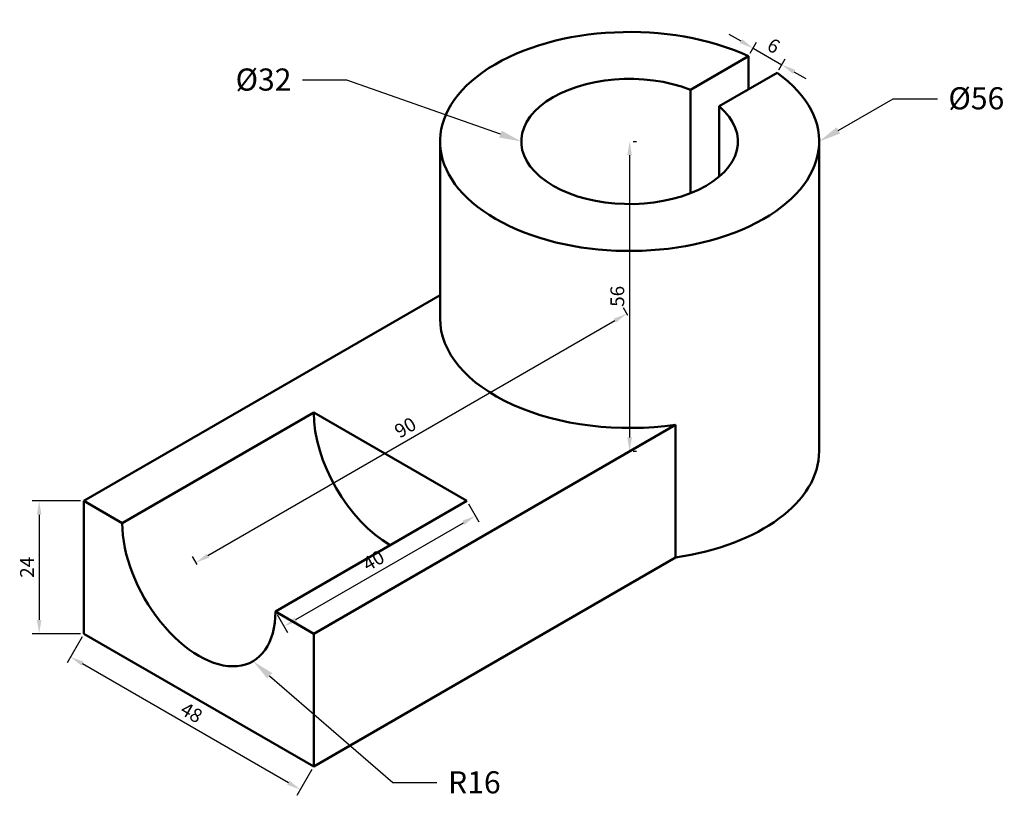
# Model space of a CAD drawing. Units: millimetres. Extents: x 2143 to 2321, y 1231 to 1373.
import ezdxf
from ezdxf import colors
from ezdxf.entities.mleader import LeaderData, LeaderLine
from ezdxf.math import Vec2, Vec3

# ---------------------------------------------------------------- set-up
doc = ezdxf.new("R2010")
doc.units = ezdxf.units.MM
for name, color, linetype, lineweight in [('M-DIMS', 2, 'Continuous', 25), ('M-OUTL', 7, 'Continuous', 50), ('M-TEXT', 3, 'Continuous', 25)]:
    doc.layers.add(name, color=color, linetype=linetype, lineweight=lineweight)
doc.styles.get("Standard").update_dxf_attribs({"font": 'arial.ttf'})
doc.dimstyles.new('ISO-25', dxfattribs={"dimtxt": 2.5, "dimasz": 2.5, "dimexe": 1.25, "dimexo": 0.625, "dimtad": 1, "dimtxsty": 'Standard', "dimcen": 2.5, "dimadec": 0, "dimazin": 0, "dimtfac": 1, "dimtmove": 0, "dimatfit": 3, "dimfxl": 1, "dimarcsym": 0})

# ---------------------------------------------------------------- blocks, each defined once
blk = doc.blocks.new('*D1')
at = {"layer": 'Defpoints', "color": 0, "transparency": 16777216}
for p in [(2154.59, 1261.56), (2152.18, 1257.37), (2196.16, 1237.56)]:
    blk.add_point(p, dxfattribs=at)
at = {"layer": 'M-DIMS', "color": 0, "lineweight": -2, "transparency": 16777216}
for p, q in [((2154.28, 1261.02), (2151.55, 1256.29)), ((2191.58, 1234.62), (2154.34, 1256.12)), ((2195.85, 1237.02), (2193.12, 1232.29))]:
    blk.add_line(p, q, dxfattribs=at)
at = {"layer": 'M-DIMS', "color": 0, "transparency": 16777216}
for points in [[(2154.55, 1256.49), (2154.14, 1255.76), (2152.18, 1257.37)], [(2191.79, 1234.99), (2191.37, 1234.26), (2193.75, 1233.37)]]:
    blk.add_solid(points, dxfattribs=at)
at = {"layer": 'M-DIMS', "color": 0, "transparency": 16777216, "insert": (2173.91, 1247.02), "char_height": 2.5, "attachment_point": 5, "rotation": 330}
blk.add_mtext('48', dxfattribs=at)
blk = doc.blocks.new('*D2')
at = {"layer": 'Defpoints', "color": 0, "transparency": 16777216}
for p in [(2223.88, 1285.56), (2225.42, 1282.87), (2189.23, 1265.56)]:
    blk.add_point(p, dxfattribs=at)
at = {"layer": 'M-DIMS', "color": 0, "lineweight": -2, "transparency": 16777216}
for p, q in [((2224.19, 1285.02), (2226.05, 1281.79)), ((2192.95, 1264.12), (2223.26, 1281.62)), ((2189.55, 1265.02), (2191.41, 1261.79))]:
    blk.add_line(p, q, dxfattribs=at)
at = {"layer": 'M-DIMS', "color": 0, "transparency": 16777216}
for points in [[(2223.05, 1281.98), (2223.47, 1281.26), (2225.42, 1282.87)], [(2192.74, 1264.48), (2193.16, 1263.76), (2190.78, 1262.87)]]:
    blk.add_solid(points, dxfattribs=at)
at = {"layer": 'M-DIMS', "color": 0, "transparency": 16777216, "insert": (2207.15, 1274.52), "char_height": 2.5, "attachment_point": 5, "rotation": 30}
blk.add_mtext('40', dxfattribs=at)
blk = doc.blocks.new('*D3')
at = {"layer": 'Defpoints', "color": 0, "transparency": 16777216}
for p in [(2154.59, 1285.56), (2146.5, 1261.56), (2154.59, 1261.56)]:
    blk.add_point(p, dxfattribs=at)
at = {"layer": 'M-DIMS', "color": 0, "lineweight": -2, "transparency": 16777216}
for p, q in [((2153.97, 1285.56), (2145.25, 1285.56)), ((2146.5, 1283.06), (2146.5, 1264.06)), ((2153.97, 1261.56), (2145.25, 1261.56))]:
    blk.add_line(p, q, dxfattribs=at)
at = {"layer": 'M-DIMS', "color": 0, "transparency": 16777216}
for points in [[(2146.08, 1283.06), (2146.91, 1283.06), (2146.5, 1285.56)], [(2146.08, 1264.06), (2146.91, 1264.06), (2146.5, 1261.56)]]:
    blk.add_solid(points, dxfattribs=at)
at = {"layer": 'M-DIMS', "color": 0, "transparency": 16777216, "insert": (2144.62, 1273.56), "char_height": 2.5, "attachment_point": 5, "rotation": 90}
blk.add_mtext('24', dxfattribs=at)
blk = doc.blocks.new('*D4')
at = {"layer": 'Defpoints', "color": 0, "transparency": 16777216}
for p in [(2252.82, 1319.42), (2253.32, 1318.56), (2175.38, 1273.56)]:
    blk.add_point(p, dxfattribs=at)
at = {"layer": 'M-DIMS', "color": 0, "lineweight": -2, "transparency": 16777216}
for p, q in [((2253.01, 1319.1), (2252.19, 1320.51)), ((2177.04, 1275.67), (2250.65, 1318.17)), ((2175.07, 1274.1), (2174.25, 1275.51))]:
    blk.add_line(p, q, dxfattribs=at)
at = {"layer": 'M-DIMS', "color": 0, "transparency": 16777216}
for points in [[(2250.45, 1318.53), (2250.86, 1317.81), (2252.82, 1319.42)], [(2176.83, 1276.03), (2177.25, 1275.31), (2174.88, 1274.42)]]:
    blk.add_solid(points, dxfattribs=at)
at = {"layer": 'M-DIMS', "color": 0, "transparency": 16777216, "insert": (2212.9, 1298.57), "char_height": 2.5, "attachment_point": 5, "rotation": 30}
blk.add_mtext('90', dxfattribs=at)
blk = doc.blocks.new('*D5')
at = {"layer": 'Defpoints', "color": 0, "transparency": 16777216}
for p in [(2253.32, 1350.56), (2253.32, 1294.56), (2253.32, 1294.56)]:
    blk.add_point(p, dxfattribs=at)
at = {"layer": 'M-DIMS', "color": 0, "lineweight": -2, "transparency": 16777216}
for p, q in [((2253.95, 1350.56), (2254.57, 1350.56)), ((2253.32, 1348.06), (2253.32, 1297.06)), ((2253.95, 1294.56), (2254.57, 1294.56))]:
    blk.add_line(p, q, dxfattribs=at)
at = {"layer": 'M-DIMS', "color": 0, "transparency": 16777216}
for points in [[(2252.9, 1348.06), (2253.74, 1348.06), (2253.32, 1350.56)], [(2252.9, 1297.06), (2253.74, 1297.06), (2253.32, 1294.56)]]:
    blk.add_solid(points, dxfattribs=at)
at = {"layer": 'M-DIMS', "color": 0, "transparency": 16777216, "insert": (2251.42, 1322.56), "char_height": 2.5, "attachment_point": 5, "rotation": 90}
blk.add_mtext('56', dxfattribs=at)
blk = doc.blocks.new('*D6')
at = {"layer": 'Defpoints', "color": 0, "transparency": 16777216}
for p in [(2274.83, 1365.98), (2280.03, 1362.98), (2280.87, 1364.43)]:
    blk.add_point(p, dxfattribs=at)
at = {"layer": 'M-DIMS', "color": 0, "lineweight": -2, "transparency": 16777216}
for p, q in [((2273.51, 1368.68), (2271.34, 1369.93)), ((2275.14, 1366.52), (2276.3, 1368.51)), ((2275.67, 1367.43), (2280.87, 1364.43)), ((2280.34, 1363.52), (2281.49, 1365.51)), ((2283.03, 1363.18), (2285.2, 1361.93))]:
    blk.add_line(p, q, dxfattribs=at)
at = {"layer": 'M-DIMS', "color": 0, "transparency": 16777216}
for points in [[(2273.71, 1369.04), (2273.3, 1368.32), (2275.67, 1367.43)], [(2283.24, 1363.54), (2282.82, 1362.82), (2280.87, 1364.43)]]:
    blk.add_solid(points, dxfattribs=at)
at = {"layer": 'M-DIMS', "color": 0, "transparency": 16777216, "insert": (2279.22, 1367.58), "char_height": 2.5, "attachment_point": 5, "rotation": 330}
blk.add_mtext('6', dxfattribs=at)

msp = doc.modelspace()

# ---------------------------------------------------------------- linework, layer by layer
at = {"layer": 'M-OUTL'}
for p, q in [((2264.333, 1359.915), (2274.831, 1365.977)), ((2274.832, 1359.977), (2274.832, 1365.977)), ((2280.027, 1362.977), (2269.529, 1356.915)), ((2264.333, 1359.915), (2264.333, 1341.199)), ((2269.529, 1356.915), (2269.529, 1344.199)), ((2219.027, 1350.557), (2219.027, 1318.557)), ((2287.613, 1350.557), (2287.613, 1294.557)), ((2219.027, 1322.758), (2154.593, 1285.557)), ((2161.521, 1281.557), (2196.162, 1301.557)), ((2196.162, 1301.557), (2223.875, 1285.557)), ((2196.162, 1261.557), (2261.615, 1299.346)), ((2261.616, 1275.346), (2261.616, 1299.346)), ((2154.593, 1285.557), (2161.521, 1281.557)), ((2154.593, 1285.557), (2154.593, 1261.557)), ((2189.234, 1265.557), (2223.875, 1285.557)), ((2196.162, 1237.557), (2261.615, 1275.346)), ((2189.234, 1265.557), (2196.162, 1261.557)), ((2154.593, 1261.557), (2196.162, 1237.557)), ((2196.162, 1237.557), (2196.162, 1261.557))]:
    msp.add_line(p, q, dxfattribs=at)
for centre, major_axis, start_param, end_param in [((2253.32, 1350.557), (-34.293, 0), 4.0343397, 10.1028272), ((2253.32, 1350.557), (-19.596, 0), 4.1156072, 10.0215597), ((2253.32, 1318.557), (-34.293, 0), 6.2831853, 8.0982803), ((2210.019, 1293.557), (9.798, -16.971), 3.9269908, 5.4977871), ((2253.32, 1294.557), (-34.293, 0), 8.0982803, 9.424778), ((2175.378, 1273.557), (9.798, -16.971), 3.9269908, 7.0685835)]:
    msp.add_ellipse(centre, major_axis=major_axis, ratio=0.5773503, start_param=start_param, end_param=end_param, dxfattribs=at)

# ---------------------------------------------------------------- dimensions: what is measured, and where the dimension line sits
at = {"layer": 'M-DIMS'}
for p1, p2, distance, picture, middle in [((2274.831, 1365.977), (2280.027, 1362.977), 1.68, '*D6', (2279.22, 1367.578)), ((2253.32, 1350.557), (2253.32, 1294.557), 0, '*D5', (2251.419, 1322.557)), ((2175.378, 1273.557), (2253.32, 1318.557), 1, '*D4', (2212.898, 1298.57)), ((2154.593, 1285.557), (2154.593, 1261.557), -8.097, '*D3', (2144.616, 1273.557)), ((2189.234, 1265.557), (2223.875, 1285.557), -3.098, '*D2', (2207.153, 1274.521)), ((2196.162, 1237.557), (2154.593, 1261.557), 4.829, '*D1', (2173.914, 1247.022))]:
    dim = msp.add_aligned_dim(p1=p1, p2=p2, distance=distance, dimstyle='ISO-25', override={"dimclrd": 0, "dimclre": 0, "dimclrt": 0}, dxfattribs=at)
    dim.commit()
    dim.dimension.update_dxf_attribs({"geometry": picture, "text_midpoint": middle})

# ---------------------------------------------------------------- leaders
at = {"layer": 'M-TEXT'}
ml = msp.add_multileader_mtext('Standard', dxfattribs=at)
ml.set_content('%%C32', color=256)
ml.set_leader_properties()
ml.build(insert=Vec2(0, 0))
ctx = ml.context
ctx.base_point, ctx.plane_origin = Vec3(2180.103, 1361.674), Vec3(2233.724, 1350.557)
ctx.text_align_type = 2
notes = []
notes.append((ctx, [(0, (1, 1, 0), (2202.144, 1361.674), (-1, 0), 8, [(0, [(2233.724, 1350.557)], 0, [])])]))
ctx.mtext.insert, ctx.mtext.alignment, ctx.mtext.flow_direction = Vec3(2192.144, 1363.755), 3, 5
ml = msp.add_multileader_mtext('Standard', dxfattribs=at)
ml.set_content('%%C56', color=256)
ml.set_leader_properties()
ml.build(insert=Vec2(0, 0))
ctx = ml.context
ctx.base_point, ctx.plane_origin = Vec3(2309.001, 1358.287), Vec3(2287.613, 1350.557)
notes.append((ctx, [(0, (1, 1, 0), (2301.001, 1358.287), (1, 0), 8, [(0, [(2287.613, 1350.557)], 0, [])])]))
ctx.mtext.insert, ctx.mtext.flow_direction = Vec3(2311.001, 1360.367), 5
ml = msp.add_multileader_mtext('Standard', dxfattribs=at)
ml.set_content('R16', color=256)
ml.set_leader_properties()
ml.build(insert=Vec2(0, 0))
ctx = ml.context
ctx.base_point, ctx.plane_origin = Vec3(2218.469, 1234.654), Vec3(2185.176, 1256.587)
notes.append((ctx, [(0, (1, 1, 0), (2210.469, 1234.654), (1, 0), 8, [(0, [(2185.176, 1256.587)], 0, [])])]))
ctx.mtext.insert, ctx.mtext.flow_direction = Vec3(2220.469, 1236.688), 5
for ctx, leaders in notes:
    for number, flags, end, landing, length, lines in leaders:
        leader = LeaderData()
        leader.index, (leader.has_last_leader_line, leader.has_dogleg_vector, leader.attachment_direction) = number, flags
        leader.last_leader_point, leader.dogleg_vector, leader.dogleg_length = Vec3(end), Vec3(landing), length
        for number, points, colour, breaks in lines:
            line = LeaderLine()
            line.index, line.vertices, line.color, line.breaks = number, Vec3.list(points), colors.encode_raw_color(colour), breaks
            leader.lines.append(line)
        ctx.leaders.append(leader)

doc.saveas('drawing.dxf')
